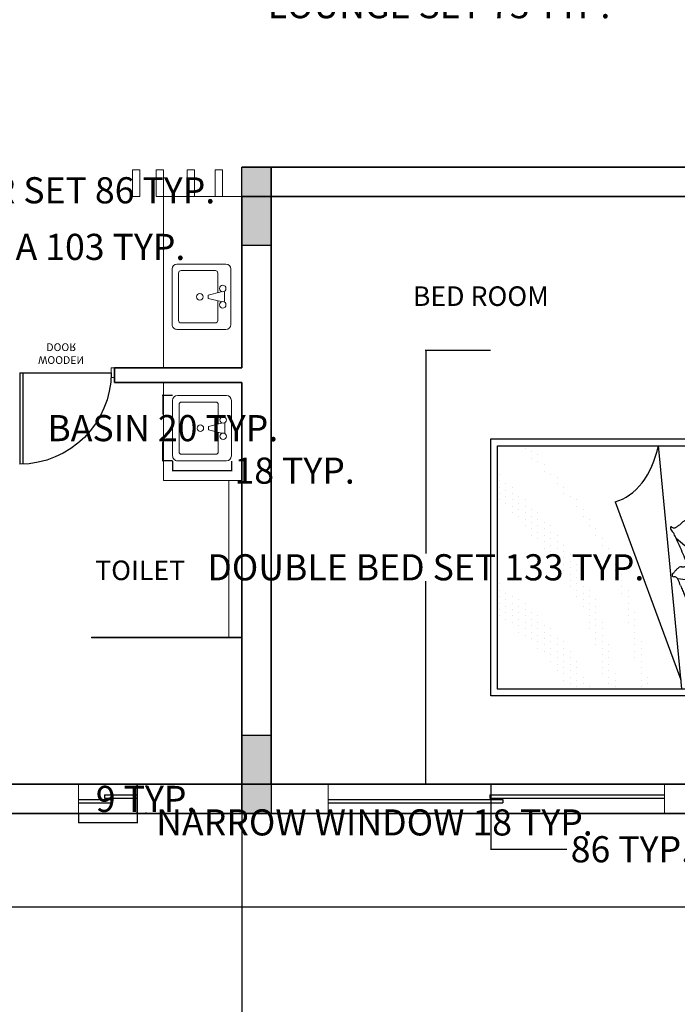
# Model space of a CAD drawing. Units: inches. Extents: x -48 to 50072, y 0 to 21068.
# Tile 63 of 75: x 974 to 1176, y 501 to 803. Entities that reach past the tile are written whole.
import ezdxf

# ---------------------------------------------------------------- set-up
doc = ezdxf.new("R2010")
doc.units = ezdxf.units.IN
doc.header["$MEASUREMENT"] = 0
for name, color, linetype, lineweight in [('A-ANNO-DIMS', 2, 'Continuous', 18), ('A-AREA-IDEN', 7, 'Continuous', 18), ('A-COLS', 1, 'Continuous', 35), ('A-DOOR', 4, 'Continuous', 18), ('A-FLOR-CASE', 9, 'Continuous', 18), ('A-FLOR-FIXT', 4, 'Continuous', 18), ('A-FLOR-SCRN', 32, 'Continuous', 18), ('A-GLAZ', 4, 'Continuous', 18), ('A-WALL', 7, 'Continuous', 35), ('FURNITURE', 44, 'Continuous', 18)]:
    doc.layers.add(name, color=color, linetype=linetype, lineweight=lineweight)
doc.layers.add('Layer3', color=176, linetype='Continuous')
doc.styles.get("Standard").update_dxf_attribs({"font": 'arial.ttf'})
doc.dimstyles.get("Standard").update_dxf_attribs({"dimtxt": 8, "dimasz": 0.18, "dimexe": 0.18, "dimexo": 0.0625, "dimgap": 0.09, "dimtad": 0, "dimtih": 1, "dimtoh": 1, "dimdec": 1, "dimzin": 0, "dimdsep": 46, "dimlunit": 4, "dimtxsty": 'Standard', "dimblk": 'ARCHTICK', "dimcen": 0.09, "dimadec": 0, "dimazin": 0, "dimtfac": 1, "dimtdec": 1, "dimtofl": 0, "dimtmove": 0, "dimatfit": 3, "dimldrblk": 'ARCHTICK', "dimfxl": 1, "dimtolj": 1, "dimtzin": 0, "dimarcsym": 0})

# ---------------------------------------------------------------- blocks, each defined once
blk = doc.blocks.new('bnniku')
at = {"layer": 'Defpoints'}
h = blk.add_hatch(color=256, dxfattribs=at)
h.dxf.hatch_style = 1
h.paths.add_polyline_path([(767.55, 1114.04), (758.55, 1114.04), (758.55, 1090.04), (767.55, 1090.04)])
for p, q in [((758.55, 1114.04), (767.55, 1114.04)), ((758.55, 1090.04), (758.55, 1114.04)), ((767.55, 1114.04), (767.55, 1090.04)), ((767.55, 1090.04), (758.55, 1090.04))]:
    blk.add_line(p, q, dxfattribs=at)
blk = doc.blocks.new('gthyerhy')
at = {"layer": 'Defpoints'}
for p, q in [((665.59, 603.33), (665.59, 631.33)), ((666.59, 603.33), (666.59, 631.32)), ((665.59, 603.33), (693.59, 603.33))]:
    blk.add_line(p, q, dxfattribs=at)
blk.add_arc((665.59, 603.33), 28, 0, 90, dxfattribs=at)
at = {"insert": (674.82, 600.63), "char_height": 2.3647, "attachment_point": 1}
blk.add_mtext_dynamic_manual_height_columns('\\pxqc;WOODEN ^JDOOR', width=6.8949, gutter_width=11.82, heights=[0], dxfattribs=at)
blk = doc.blocks.new('jyugcli')
for p, q in [((342.02, 1025.77), (342.02, 1034.77)), ((360.02, 1025.77), (360.02, 1034.77))]:
    blk.add_line(p, q)
at = {"layer": 'Defpoints'}
for p, q in [((350.02, 1031.47), (360.02, 1031.47)), ((350.02, 1031.47), (350.02, 1030.47)), ((342.02, 1030.07), (352.02, 1030.07)), ((342.02, 1029.07), (352.02, 1029.07)), ((350.02, 1030.47), (360.02, 1030.47)), ((352.02, 1030.07), (352.02, 1029.07))]:
    blk.add_line(p, q, dxfattribs=at)
at = {"layer": 'Layer3'}
for p, q in [((342.02, 1034.77), (360.02, 1034.77)), ((342.02, 1025.77), (360.02, 1025.77))]:
    blk.add_line(p, q, dxfattribs=at)
blk = doc.blocks.new('fdsghhhhhhygr')
for p, q in [((41.77, 686.77), (41.77, 677.77)), ((144.77, 677.77), (144.77, 686.77))]:
    blk.add_line(p, q)
at = {"layer": 'Defpoints'}
for p, q in [((41.77, 682.07), (95.27, 682.07)), ((91.27, 683.47), (144.77, 683.47)), ((91.27, 683.47), (91.27, 682.47)), ((91.27, 682.47), (144.77, 682.47)), ((95.27, 682.07), (95.27, 681.07)), ((41.77, 681.07), (95.27, 681.07))]:
    blk.add_line(p, q, dxfattribs=at)
at = {"layer": 'Layer3'}
for p, q in [((41.77, 686.77), (144.77, 686.77)), ((144.77, 677.77), (41.77, 677.77))]:
    blk.add_line(p, q, dxfattribs=at)
blk = doc.blocks.new('nhrygfdu7yu')
at = {"layer": 'Defpoints'}
for p, q in [((1019.17, 828.61), (845.97, 828.61)), ((845.97, 801.61), (845.97, 828.61)), ((848.67, 804.31), (848.67, 828.61)), ((881.27, 716.83), (881.27, 828.61)), ((884.03, 719.53), (884.03, 827.53)), ((884.03, 827.53), (981.17, 827.53)), ((981.17, 827.53), (981.17, 719.53)), ((983.87, 828.61), (983.87, 716.83)), ((1000.24, 805.98), (1000.24, 825.78)), ((1016.47, 804.31), (1016.47, 828.61)), ((1019.17, 801.61), (1019.17, 828.61)), ((864.18, 805.04), (864.18, 824.84)), ((892.12, 822.13), (892.12, 801.97)), ((929.67, 822.13), (892.12, 822.13)), ((929.67, 822.13), (929.67, 801.78)), ((935.52, 822.13), (935.52, 801.78)), ((935.52, 822.13), (973.07, 822.13)), ((973.07, 822.13), (973.07, 801.97)), ((926.47, 818.07), (927.21, 812.5)), ((947.88, 818.06), (943.61, 812.45)), ((874.65, 814.99), (853.09, 814.99)), ((1010.72, 815.93), (989.15, 815.93)), ((914.58, 810.18), (913.28, 809.99)), ((919.69, 808.14), (914.58, 810.18)), ((927.21, 812.5), (925.82, 805.91)), ((934.43, 807.75), (933.36, 812.55)), ((943.61, 812.45), (939.55, 805.41)), ((923.4, 803.12), (919.69, 808.14)), ((935.49, 804.66), (934.43, 807.75)), ((881.07, 804.31), (848.67, 804.31)), ((881.07, 804.31), (881.07, 804.31)), ((910.77, 803.49), (910.59, 803.15)), ((916.07, 804.42), (910.77, 803.49)), ((919.78, 804.61), (916.07, 804.42)), ((923.4, 803.12), (919.78, 804.61)), ((925.82, 805.91), (923.4, 803.12)), ((923.4, 803.12), (925.08, 798.67)), ((923.4, 803.12), (933.44, 802.1)), ((933.44, 802.1), (936.13, 800.15)), ((935.45, 803.17), (936.69, 800.13)), ((938.59, 802.42), (935.49, 804.66)), ((938.59, 802.42), (937.95, 797.34)), ((939.55, 805.41), (938.59, 802.42)), ((938.59, 802.42), (945.53, 804.13)), ((938.59, 802.42), (941.26, 799.01)), ((945.53, 804.13), (951.08, 803.38)), ((951.08, 803.38), (953.02, 802.3)), ((984.07, 804.31), (1016.47, 804.31)), ((984.07, 804.31), (984.07, 804.31)), ((881.07, 801.61), (845.97, 801.61)), ((884.06, 801.97), (981.18, 801.97)), ((925.08, 798.67), (923.96, 794.21)), ((936.13, 800.15), (936.78, 799.69)), ((936.69, 800.13), (937.65, 797.78)), ((941.26, 799.01), (944.78, 796.45)), ((984.07, 801.61), (1019.17, 801.61)), ((923.96, 794.21), (921.07, 790.83)), ((937.86, 796.54), (937.22, 791.44)), ((944.78, 796.45), (949.8, 796.45)), ((981.13, 793.06), (883.98, 783.7)), ((906.36, 766.47), (977.44, 792.73)), ((976.41, 779.36), (976.41, 779.36)), ((978.98, 779.36), (978.98, 779.36)), ((962.27, 776.79), (962.27, 776.79)), ((964.84, 776.79), (964.84, 776.79)), ((967.41, 776.79), (967.41, 776.79)), ((969.98, 776.79), (969.98, 776.79)), ((972.55, 776.79), (972.55, 776.79)), ((975.13, 776.79), (975.13, 776.79)), ((977.7, 776.79), (977.7, 776.79)), ((980.27, 776.79), (980.27, 776.79)), ((941.69, 771.64), (941.69, 771.64)), ((944.27, 771.64), (944.27, 771.64)), ((946.84, 771.64), (946.84, 771.64)), ((949.41, 771.64), (949.41, 771.64)), ((950.69, 774.21), (950.69, 774.21)), ((951.98, 771.64), (951.98, 771.64)), ((953.27, 774.21), (953.27, 774.21)), ((954.55, 771.64), (954.55, 771.64)), ((955.84, 774.21), (955.84, 774.21)), ((958.41, 774.21), (958.41, 774.21)), ((960.98, 774.21), (960.98, 774.21)), ((963.55, 774.21), (963.55, 774.21)), ((966.13, 774.21), (966.13, 774.21)), ((968.7, 774.21), (968.7, 774.21)), ((935.26, 769.07), (935.26, 769.07)), ((937.84, 769.07), (937.84, 769.07)), ((940.41, 769.07), (940.41, 769.07)), ((942.98, 769.07), (942.98, 769.07)), ((924.98, 763.93), (924.98, 763.93)), ((927.55, 763.93), (927.55, 763.93)), ((928.83, 766.5), (928.83, 766.5)), ((930.12, 763.93), (930.12, 763.93)), ((931.41, 766.5), (931.41, 766.5)), ((933.98, 766.5), (933.98, 766.5)), ((936.55, 766.5), (936.55, 766.5)), ((963.55, 763.93), (963.55, 763.93)), ((966.13, 763.93), (966.13, 763.93)), ((968.7, 763.93), (968.7, 763.93)), ((971.27, 763.93), (971.27, 763.93)), ((973.84, 763.93), (973.84, 763.93)), ((975.13, 766.5), (975.13, 766.5)), ((976.41, 763.93), (976.41, 763.93)), ((977.7, 766.5), (977.7, 766.5)), ((978.98, 763.93), (978.98, 763.93)), ((980.27, 766.5), (980.27, 766.5)), ((921.12, 761.35), (921.12, 761.35)), ((923.69, 761.35), (923.69, 761.35)), ((954.55, 761.35), (954.55, 761.35)), ((957.12, 761.35), (957.12, 761.35)), ((959.7, 761.35), (959.7, 761.35)), ((962.27, 761.35), (962.27, 761.35)), ((964.84, 761.35), (964.84, 761.35)), ((967.41, 761.35), (967.41, 761.35)), ((969.98, 761.35), (969.98, 761.35)), ((972.55, 761.35), (972.55, 761.35)), ((975.13, 761.35), (975.13, 761.35)), ((913.4, 756.21), (913.4, 756.21)), ((915.98, 756.21), (915.98, 756.21)), ((917.26, 758.78), (917.26, 758.78)), ((919.83, 758.78), (919.83, 758.78)), ((941.69, 756.21), (941.69, 756.21)), ((944.27, 756.21), (944.27, 756.21)), ((945.55, 758.78), (945.55, 758.78)), ((946.84, 756.21), (946.84, 756.21)), ((948.12, 758.78), (948.12, 758.78)), ((949.41, 756.21), (949.41, 756.21)), ((950.69, 758.78), (950.69, 758.78)), ((951.98, 756.21), (951.98, 756.21)), ((953.27, 758.78), (953.27, 758.78)), ((954.55, 756.21), (954.55, 756.21)), ((955.84, 758.78), (955.84, 758.78)), ((957.12, 756.21), (957.12, 756.21)), ((958.41, 758.78), (958.41, 758.78)), ((960.98, 758.78), (960.98, 758.78)), ((963.55, 758.78), (963.55, 758.78)), ((980.27, 756.21), (980.27, 756.21)), ((905.69, 751.07), (905.69, 751.07)), ((908.26, 751.07), (908.26, 751.07)), ((909.55, 753.64), (909.55, 753.64)), ((912.12, 753.64), (912.12, 753.64)), ((931.41, 751.07), (931.41, 751.07)), ((933.98, 751.07), (933.98, 751.07)), ((935.26, 753.64), (935.26, 753.64)), ((936.55, 751.07), (936.55, 751.07)), ((937.84, 753.64), (937.84, 753.64)), ((939.12, 751.07), (939.12, 751.07)), ((940.41, 753.64), (940.41, 753.64)), ((941.69, 751.07), (941.69, 751.07)), ((942.98, 753.64), (942.98, 753.64)), ((944.27, 751.07), (944.27, 751.07)), ((945.55, 753.64), (945.55, 753.64)), ((948.12, 753.64), (948.12, 753.64)), ((969.98, 751.07), (969.98, 751.07)), ((972.55, 751.07), (972.55, 751.07)), ((975.13, 751.07), (975.13, 751.07)), ((976.41, 753.64), (976.41, 753.64)), ((977.7, 751.07), (977.7, 751.07)), ((978.98, 753.64), (978.98, 753.64)), ((980.27, 751.07), (980.27, 751.07)), ((904.4, 748.5), (904.4, 748.5)), ((927.55, 748.5), (927.55, 748.5)), ((930.12, 748.5), (930.12, 748.5)), ((932.69, 748.5), (932.69, 748.5)), ((935.26, 748.5), (935.26, 748.5)), ((937.84, 748.5), (937.84, 748.5)), ((940.41, 748.5), (940.41, 748.5)), ((966.13, 748.5), (966.13, 748.5)), ((968.7, 748.5), (968.7, 748.5)), ((971.27, 748.5), (971.27, 748.5)), ((973.84, 748.5), (973.84, 748.5)), ((976.41, 748.5), (976.41, 748.5)), ((978.98, 748.5), (978.98, 748.5)), ((896.69, 743.35), (896.69, 743.35)), ((899.26, 743.35), (899.26, 743.35)), ((900.55, 745.92), (900.55, 745.92)), ((903.12, 745.92), (903.12, 745.92)), ((919.83, 743.35), (919.83, 743.35)), ((922.41, 743.35), (922.41, 743.35)), ((923.69, 745.92), (923.69, 745.92)), ((924.98, 743.35), (924.98, 743.35)), ((926.26, 745.92), (926.26, 745.92)), ((927.55, 743.35), (927.55, 743.35)), ((928.83, 745.92), (928.83, 745.92)), ((930.12, 743.35), (930.12, 743.35)), ((931.41, 745.92), (931.41, 745.92)), ((932.69, 743.35), (932.69, 743.35)), ((933.98, 745.92), (933.98, 745.92)), ((960.98, 743.35), (960.98, 743.35)), ((962.27, 745.92), (962.27, 745.92)), ((963.55, 743.35), (963.55, 743.35)), ((964.84, 745.92), (964.84, 745.92)), ((966.13, 743.35), (966.13, 743.35)), ((967.41, 745.92), (967.41, 745.92)), ((968.7, 743.35), (968.7, 743.35)), ((969.98, 745.92), (969.98, 745.92)), ((971.27, 743.35), (971.27, 743.35)), ((972.55, 745.92), (972.55, 745.92)), ((973.84, 743.35), (973.84, 743.35)), ((975.13, 745.92), (975.13, 745.92)), ((977.7, 745.92), (977.7, 745.92)), ((895.4, 740.78), (895.4, 740.78)), ((915.98, 740.78), (915.98, 740.78)), ((918.55, 740.78), (918.55, 740.78)), ((921.12, 740.78), (921.12, 740.78)), ((923.69, 740.78), (923.69, 740.78)), ((926.26, 740.78), (926.26, 740.78)), ((928.83, 740.78), (928.83, 740.78)), ((957.12, 740.78), (957.12, 740.78)), ((959.7, 740.78), (959.7, 740.78)), ((962.27, 740.78), (962.27, 740.78)), ((964.84, 740.78), (964.84, 740.78)), ((967.41, 740.78), (967.41, 740.78)), ((969.98, 740.78), (969.98, 740.78)), ((887.69, 735.64), (887.69, 735.64)), ((890.26, 735.64), (890.26, 735.64)), ((891.54, 738.21), (891.54, 738.21)), ((894.12, 738.21), (894.12, 738.21)), ((910.83, 735.64), (910.83, 735.64)), ((913.4, 735.64), (913.4, 735.64)), ((914.69, 738.21), (914.69, 738.21)), ((915.98, 735.64), (915.98, 735.64)), ((917.26, 738.21), (917.26, 738.21)), ((918.55, 735.64), (918.55, 735.64)), ((919.83, 738.21), (919.83, 738.21)), ((921.12, 735.64), (921.12, 735.64)), ((922.41, 738.21), (922.41, 738.21)), ((924.98, 738.21), (924.98, 738.21)), ((951.98, 735.64), (951.98, 735.64)), ((954.55, 735.64), (954.55, 735.64)), ((955.84, 738.21), (955.84, 738.21)), ((957.12, 735.64), (957.12, 735.64)), ((958.41, 738.21), (958.41, 738.21)), ((959.7, 735.64), (959.7, 735.64)), ((960.98, 738.21), (960.98, 738.21)), ((962.27, 735.64), (962.27, 735.64)), ((963.55, 738.21), (963.55, 738.21)), ((964.84, 735.64), (964.84, 735.64)), ((966.13, 738.21), (966.13, 738.21)), ((886.4, 733.07), (886.4, 733.07)), ((888.97, 733.07), (888.97, 733.07)), ((909.55, 733.07), (909.55, 733.07)), ((912.12, 733.07), (912.12, 733.07)), ((914.69, 733.07), (914.69, 733.07)), ((917.26, 733.07), (917.26, 733.07)), ((919.83, 733.07), (919.83, 733.07)), ((950.69, 733.07), (950.69, 733.07)), ((953.27, 733.07), (953.27, 733.07)), ((955.84, 733.07), (955.84, 733.07)), ((958.41, 733.07), (958.41, 733.07)), ((960.98, 733.07), (960.98, 733.07)), ((885.12, 730.49), (885.12, 730.49)), ((904.4, 727.92), (904.4, 727.92)), ((905.69, 730.49), (905.69, 730.49)), ((906.97, 727.92), (906.97, 727.92)), ((908.26, 730.49), (908.26, 730.49)), ((909.55, 727.92), (909.55, 727.92)), ((910.83, 730.49), (910.83, 730.49)), ((912.12, 727.92), (912.12, 727.92)), ((913.4, 730.49), (913.4, 730.49)), ((915.98, 730.49), (915.98, 730.49)), ((945.55, 727.92), (945.55, 727.92)), ((946.84, 730.49), (946.84, 730.49)), ((948.12, 727.92), (948.12, 727.92)), ((949.41, 730.49), (949.41, 730.49)), ((950.69, 727.92), (950.69, 727.92)), ((951.98, 730.49), (951.98, 730.49)), ((953.27, 727.92), (953.27, 727.92)), ((954.55, 730.49), (954.55, 730.49)), ((955.84, 727.92), (955.84, 727.92)), ((957.12, 730.49), (957.12, 730.49)), ((958.41, 727.92), (958.41, 727.92)), ((959.7, 730.49), (959.7, 730.49)), ((900.55, 725.35), (900.55, 725.35)), ((903.12, 725.35), (903.12, 725.35)), ((905.69, 725.35), (905.69, 725.35)), ((908.26, 725.35), (908.26, 725.35)), ((910.83, 725.35), (910.83, 725.35)), ((944.27, 725.35), (944.27, 725.35)), ((946.84, 725.35), (946.84, 725.35)), ((949.41, 725.35), (949.41, 725.35)), ((951.98, 725.35), (951.98, 725.35)), ((954.55, 725.35), (954.55, 725.35)), ((981.17, 719.53), (884.03, 719.53)), ((895.4, 720.21), (895.4, 720.21)), ((897.97, 720.21), (897.97, 720.21)), ((899.26, 722.78), (899.26, 722.78)), ((900.55, 720.21), (900.55, 720.21)), ((901.83, 722.78), (901.83, 722.78)), ((903.12, 720.21), (903.12, 720.21)), ((904.4, 722.78), (904.4, 722.78)), ((905.69, 720.21), (905.69, 720.21)), ((906.97, 722.78), (906.97, 722.78)), ((939.12, 720.21), (939.12, 720.21)), ((941.69, 720.21), (941.69, 720.21)), ((942.98, 722.78), (942.98, 722.78)), ((944.27, 720.21), (944.27, 720.21)), ((945.55, 722.78), (945.55, 722.78)), ((946.84, 720.21), (946.84, 720.21)), ((948.12, 722.78), (948.12, 722.78)), ((949.41, 720.21), (949.41, 720.21)), ((950.69, 722.78), (950.69, 722.78)), ((951.98, 720.21), (951.98, 720.21)), ((953.27, 722.78), (953.27, 722.78)), ((983.87, 716.83), (881.27, 716.83))]:
    blk.add_line(p, q, dxfattribs=at)
for centre, radius in [((864.18, 814.99), 8.1), ((1000.24, 815.93), 8.1), ((1000.24, 815.93), 6.48), ((864.18, 814.99), 6.48)]:
    blk.add_circle(centre, radius, dxfattribs=at)
for centre, radius, start, end in [((926.67, 817.58), 0.687, 51.1864, 183.2455), ((924.75, 815.18), 3.76, 45.8726, 51.1864), ((929.07, 819.63), 2.44, 225.8726, 232.4713), ((948.22, 814.9), 3.25, 110.3452, 128.5854), ((947.75, 816.16), 1.9, 86.0516, 110.3452), ((947.87, 817.82), 0.239, 13.2808, 86.0516), ((947.77, 817.8), 0.34, 306.5792, 13.2808), ((971.1, 717.04), 108.88, 116.4147, 117.4999), ((848.26, 964.34), 167.25, 296.4147, 297.2902), ((924.05, 817.43), 1.94, 297.2902, 3.2455), ((940.16, 834.08), 20.66, 232.4713, 233.7837), ((906.88, 788.64), 35.67, 52.7849, 53.7837), ((921.35, 807.68), 11.75, 46.4776, 52.7849), ((926.56, 813.17), 4.18, 35.8936, 46.4776), ((928.96, 814.91), 1.22, 351.9508, 35.8936), ((932.62, 814.39), 2.47, 171.9508, 202.4162), ((883.03, 974.91), 169.83, 286.6085, 289.0836), ((848.62, 1074.38), 275.09, 289.0836, 290.1287), ((927.73, 858.54), 45.2, 290.1287, 292.7069), ((943.53, 820.78), 4.28, 292.7069, 308.5854), ((951.77, 816.3), 4.17, 169.5926, 177.2714), ((948.44, 816.46), 0.826, 177.2714, 194.5709), ((949.69, 816.78), 2.12, 194.5709, 206.8179), ((948.43, 816.91), 0.765, 126.5792, 169.5926), ((964.76, 824.4), 19.01, 206.8179, 210.9056), ((957.44, 820.02), 10.47, 210.9056, 219.7005), ((905.47, 831.87), 23.22, 282.6252, 290.7486), ((901.77, 841.65), 33.68, 290.7486, 297.4921), ((771.78, 1091.44), 315.27, 297.4921, 297.8482), ((1072.97, 521.35), 329.5, 117.4999, 117.8482), ((980.52, 834.15), 54.29, 202.4162, 205.0529), ((929.77, 818.2), 6.29, 280.7366, 286.6085), ((1013.86, 849.73), 91.09, 205.0529, 207.0884), ((946.01, 810.53), 4.37, 26.0735, 39.7005), ((940.41, 807.79), 10.61, 17.8396, 26.0735), ((847.55, 777.91), 108.16, 15.2625, 17.8396), ((908.02, 808.45), 0.313, 121.6917, 179.0386), ((908.61, 808.44), 0.905, 179.0386, 229.4914), ((909.3, 806.38), 2.75, 103.0402, 121.6917), ((905.38, 804.66), 4.08, 26.3332, 49.4914), ((909.41, 805.91), 3.23, 86.6119, 103.0402), ((780.21, 742.7), 143.74, 25.1732, 26.3332), ((909.8, 812.53), 3.4, 266.6119, 282.6252), ((1008.01, 846.74), 84.52, 207.0884, 209.936), ((866.04, 782.95), 89, 13.841, 15.2625), ((901.51, 799.71), 9.71, 20.7081, 25.1732), ((883.04, 792.73), 29.45, 18.2369, 20.7081), ((924.73, 798.79), 11.57, 22.2355, 29.936), ((981.05, 811.29), 29.45, 193.841, 196.3122), ((962.1, 805.74), 9.71, 196.3122, 200.7773), ((1087.42, 853.29), 143.74, 200.7773, 201.9373), ((995.54, 829.8), 89, 198.2369, 199.6584), ((1013.59, 836.25), 108.16, 199.6584, 202.2355), ((957.87, 801.11), 4.08, 201.9373, 225.0955), ((954.35, 797.58), 0.905, 354.6428, 45.0955), ((923.29, 799.33), 10.61, 202.2355, 210.4694), ((993.31, 637.11), 169.83, 111.0043, 113.4795), ((880.68, 777.46), 54.29, 18.0203, 19.3448), ((929.96, 793.49), 2.47, 347.5549, 18.0203), ((934.7, 789.77), 6.29, 98.1216, 111.0043), ((934.31, 792.46), 3.58, 85.4882, 98.1216), ((934.9, 799.87), 3.85, 265.4882, 277.6784), ((934.12, 805.65), 9.69, 277.6784, 284.8807), ((939.32, 786.09), 10.56, 97.9822, 104.8807), ((938.8, 798.25), 1.24, 202.2355, 252.8133), ((938.1, 794.73), 1.83, 85.7407, 97.9822), ((938.28, 797.05), 0.497, 265.7407, 289.3799), ((938.36, 796.82), 0.252, 289.3799, 72.8133), ((1069.09, 504.93), 315.27, 113.0962, 113.4523), ((958.63, 763.95), 33.68, 106.3527, 113.0962), ((955.69, 773.98), 23.22, 98.2293, 106.3527), ((952.85, 793.6), 3.4, 82.216, 98.2293), ((953.75, 800.17), 3.23, 262.216, 278.6443), ((953.82, 799.69), 2.75, 278.6443, 297.2959), ((954.94, 797.53), 0.313, 297.2959, 354.6428), ((917.92, 796.17), 4.37, 210.4694, 224.0964), ((907.26, 785.84), 10.47, 35.3015, 44.0964), ((900.29, 780.91), 19.01, 31.2138, 35.3015), ((914.73, 789.66), 2.12, 18.9668, 31.2138), ((915.96, 790.08), 0.826, 1.6673, 18.9668), ((939.83, 749.71), 45.2, 114.5246, 117.1028), ((1035.25, 540.56), 275.09, 113.4795, 114.5246), ((933.57, 792.7), 1.22, 167.5549, 211.4977), ((936.09, 794.24), 4.18, 211.4977, 222.0817), ((941.71, 799.32), 11.75, 222.0817, 228.389), ((957.59, 817.2), 35.67, 228.389, 229.3878), ((938.27, 789.81), 1.94, 112.8944, 178.8496), ((1002.58, 637.52), 167.25, 112.0188, 112.8944), ((899.06, 893.51), 108.88, 292.0188, 293.104), ((812.48, 1096.43), 329.5, 293.104, 293.4523), ((916.73, 788.79), 0.34, 130.9751, 197.6767), ((916.63, 788.76), 0.239, 197.6767, 270.4475), ((916, 789.63), 0.765, 310.9751, 353.9885), ((916.62, 790.42), 1.9, 270.4475, 294.7411), ((912.62, 789.98), 4.17, 353.9885, 1.6673), ((916.05, 791.65), 3.25, 294.7411, 312.9813), ((921.18, 786.14), 4.28, 117.1028, 132.9813), ((920.93, 774.44), 20.66, 48.0754, 49.3878), ((933.1, 787.99), 2.44, 41.4767, 48.0754), ((937.75, 792.1), 3.76, 221.4767, 226.7905), ((935.64, 789.86), 0.687, 226.7905, 358.8496)]:
    blk.add_arc(centre, radius, start, end, dxfattribs=at)
blk.add_ellipse((874.1, 762.91), major_axis=(32.71, 0), ratio=0.667085, start_param=0.16392, end_param=1.263761, dxfattribs=at)
blk = doc.blocks.new('A$C329C6BD7')
at = {"linetype": 'ByBlock'}
for p, q in [((0, 0.4191), (0, 0.0381)), ((0.4699, 0.4572), (0.0381, 0.4572)), ((0.2159, 0.4064), (0.2921, 0.4064)), ((0.508, 0.0381), (0.508, 0.4191)), ((0.0508, 0.0698), (0.0508, 0.3365)), ((0.0698, 0.3556), (0.2223, 0.3556)), ((0.2159, 0.381), (0.2413, 0.2794)), ((0.2667, 0.2794), (0.2921, 0.381)), ((0.2858, 0.3556), (0.4382, 0.3556)), ((0.4572, 0.3365), (0.4572, 0.0698)), ((0.2413, 0.2794), (0.2667, 0.2794)), ((0.4382, 0.0508), (0.0698, 0.0508)), ((0.0381, 0), (0.4699, 0))]:
    blk.add_line(p, q, dxfattribs=at)
for centre in [(0.1905, 0.3937), (0.3175, 0.3937), (0.254, 0.2159)]:
    blk.add_circle(centre, 0.0254, dxfattribs=at)
for centre, radius, start, end in [((0.0381, 0.4191), 0.0381, 90, 180), ((0.4699, 0.4191), 0.0381, 0, 90), ((0.0698, 0.3365), 0.0191, 90, 180), ((0.4382, 0.3365), 0.0191, 0, 90), ((0.0381, 0.0381), 0.0381, 180, 270), ((0.0698, 0.0698), 0.0191, 180, 270), ((0.4382, 0.0698), 0.0191, 270, 0), ((0.4699, 0.0381), 0.0381, 270, 0)]:
    blk.add_arc(centre, radius, start, end, dxfattribs=at)
blk = doc.blocks.new('_ArchTick')
at = {"color": 0, "linetype": 'ByBlock', "const_width": 0.15}
blk.add_lwpolyline([(-0.5, -0.5), (0.5, 0.5)], dxfattribs=at)
blk = doc.blocks.new('*D56')
at = {"layer": 'A-ANNO-DIMS', "color": 0, "lineweight": -2, "transparency": 16777216}
for p, q in [((992.26, 559.4), (992.26, 556.58)), ((1010.26, 559.4), (1010.26, 556.58)), ((992.26, 556.76), (1010.26, 556.76)), ((1010.26, 556.76), (1010.44, 556.76))]:
    blk.add_line(p, q, dxfattribs=at)
at = {"layer": 'Defpoints', "color": 0, "transparency": 16777216}
for p in [(992.26, 559.46), (1010.26, 559.46), (1010.26, 556.76)]:
    blk.add_point(p, dxfattribs=at)
at = {"layer": 'A-ANNO-DIMS', "color": 0, "lineweight": -2, "transparency": 16777216, "xscale": 0.18, "yscale": 0.18, "zscale": 0.18, "rotation": 180}
blk.add_blockref('_ArchTick', (992.26, 556.76), dxfattribs=at)
at = {"layer": 'A-ANNO-DIMS', "color": 0, "lineweight": -2, "transparency": 16777216, "xscale": 0.18, "yscale": 0.18, "zscale": 0.18}
blk.add_blockref('_ArchTick', (1010.26, 556.76), dxfattribs=at)
at = {"layer": 'A-ANNO-DIMS', "color": 0, "transparency": 16777216, "insert": (1082.89, 556.76), "char_height": 8, "attachment_point": 5}
blk.add_mtext('\\A1;NARROW WINDOW 18 TYP.', dxfattribs=at)
blk = doc.blocks.new('*D57')
at = {"layer": 'A-ANNO-DIMS', "color": 0, "lineweight": -2, "transparency": 16777216}
for p, q in [((1010.32, 568.46), (1013.14, 568.46)), ((1012.96, 568.46), (1012.96, 568.14)), ((1010.32, 559.46), (1013.14, 559.46)), ((1012.96, 559.46), (1012.96, 559.79))]:
    blk.add_line(p, q, dxfattribs=at)
at = {"layer": 'Defpoints', "color": 0, "transparency": 16777216}
for p in [(1010.26, 568.46), (1012.96, 568.46), (1010.26, 559.46)]:
    blk.add_point(p, dxfattribs=at)
at = {"layer": 'A-ANNO-DIMS', "color": 0, "lineweight": -2, "transparency": 16777216, "xscale": 0.18, "yscale": 0.18, "zscale": 0.18}
for p, rotation in [((1012.96, 568.46), 90), ((1012.96, 559.46), 270)]:
    blk.add_blockref('_ArchTick', p, dxfattribs=dict(at, rotation=rotation))
at = {"layer": 'A-ANNO-DIMS', "color": 0, "transparency": 16777216, "insert": (1012.96, 563.96), "char_height": 8, "attachment_point": 5}
blk.add_mtext('\\A1;9 TYP.', dxfattribs=at)
blk = doc.blocks.new('*D60')
at = {"layer": 'A-ANNO-DIMS', "color": 0, "lineweight": -2, "transparency": 16777216}
for p, q in [((787.01, 748.4), (787.01, 732.83)), ((890.01, 748.4), (890.01, 732.83)), ((787.01, 733.01), (890.01, 733.01)), ((890.01, 733.01), (890.19, 733.01))]:
    blk.add_line(p, q, dxfattribs=at)
at = {"layer": 'Defpoints', "color": 0, "transparency": 16777216}
for p in [(787.01, 748.46), (890.01, 748.46), (890.01, 733.01)]:
    blk.add_point(p, dxfattribs=at)
at = {"layer": 'A-ANNO-DIMS', "color": 0, "lineweight": -2, "transparency": 16777216, "xscale": 0.18, "yscale": 0.18, "zscale": 0.18, "rotation": 180}
blk.add_blockref('_ArchTick', (787.01, 733.01), dxfattribs=at)
at = {"layer": 'A-ANNO-DIMS', "color": 0, "lineweight": -2, "transparency": 16777216, "xscale": 0.18, "yscale": 0.18, "zscale": 0.18}
blk.add_blockref('_ArchTick', (890.01, 733.01), dxfattribs=at)
at = {"layer": 'A-ANNO-DIMS', "color": 0, "transparency": 16777216, "insert": (960.35, 733.01), "char_height": 8, "attachment_point": 5}
blk.add_mtext('\\A1;SLIDING DOOR A 103 TYP.', dxfattribs=at)
blk = doc.blocks.new('*D72')
at = {"layer": 'A-ANNO-DIMS', "color": 0, "lineweight": -2, "transparency": 16777216}
for p, q in [((1118.47, 701.3), (1098.43, 701.3)), ((1098.61, 701.3), (1098.61, 639.11)), ((1098.61, 568.46), (1098.61, 630.65)), ((1118.47, 568.46), (1098.43, 568.46))]:
    blk.add_line(p, q, dxfattribs=at)
at = {"layer": 'Defpoints', "color": 0, "transparency": 16777216}
for p in [(1118.53, 701.3), (1098.61, 568.46), (1118.53, 568.46)]:
    blk.add_point(p, dxfattribs=at)
at = {"layer": 'A-ANNO-DIMS', "color": 0, "lineweight": -2, "transparency": 16777216, "xscale": 0.18, "yscale": 0.18, "zscale": 0.18}
for p, rotation in [((1098.61, 701.3), 90), ((1098.61, 568.46), 270)]:
    blk.add_blockref('_ArchTick', p, dxfattribs=dict(at, rotation=rotation))
at = {"layer": 'A-ANNO-DIMS', "color": 0, "transparency": 16777216, "insert": (1098.61, 634.88), "char_height": 8, "attachment_point": 5}
blk.add_mtext('\\A1;DOUBLE BED SET 133 TYP.', dxfattribs=at)
blk = doc.blocks.new('*D73')
at = {"layer": 'A-ANNO-DIMS', "color": 0, "lineweight": -2, "transparency": 16777216}
for p, q in [((1118.53, 568.4), (1118.53, 548.36)), ((1204.26, 568.4), (1204.26, 548.36)), ((1118.53, 548.54), (1141.83, 548.54)), ((1204.26, 548.54), (1180.96, 548.54))]:
    blk.add_line(p, q, dxfattribs=at)
at = {"layer": 'Defpoints', "color": 0, "transparency": 16777216}
for p in [(1118.53, 568.46), (1204.26, 568.46), (1204.26, 548.54)]:
    blk.add_point(p, dxfattribs=at)
at = {"layer": 'A-ANNO-DIMS', "color": 0, "lineweight": -2, "transparency": 16777216, "xscale": 0.18, "yscale": 0.18, "zscale": 0.18, "rotation": 180}
blk.add_blockref('_ArchTick', (1118.53, 548.54), dxfattribs=at)
at = {"layer": 'A-ANNO-DIMS', "color": 0, "lineweight": -2, "transparency": 16777216, "xscale": 0.18, "yscale": 0.18, "zscale": 0.18}
blk.add_blockref('_ArchTick', (1204.26, 548.54), dxfattribs=at)
at = {"layer": 'A-ANNO-DIMS', "color": 0, "transparency": 16777216, "insert": (1161.4, 548.54), "char_height": 8, "attachment_point": 5}
blk.add_mtext('\\A1;86 TYP.', dxfattribs=at)
blk = doc.blocks.new('*D76')
at = {"layer": 'A-ANNO-DIMS', "color": 0, "lineweight": -2, "transparency": 16777216}
for p, q in [((972.12, 817.98), (972.12, 806.85)), ((1045.51, 817.98), (1045.51, 806.85)), ((972.12, 807.03), (1045.51, 807.03)), ((1045.51, 807.03), (1045.69, 807.03))]:
    blk.add_line(p, q, dxfattribs=at)
at = {"layer": 'Defpoints', "color": 0, "transparency": 16777216}
for p in [(972.12, 818.04), (1045.51, 818.04), (1045.51, 807.03)]:
    blk.add_point(p, dxfattribs=at)
at = {"layer": 'A-ANNO-DIMS', "color": 0, "lineweight": -2, "transparency": 16777216, "xscale": 0.18, "yscale": 0.18, "zscale": 0.18, "rotation": 180}
blk.add_blockref('_ArchTick', (972.12, 807.03), dxfattribs=at)
at = {"layer": 'A-ANNO-DIMS', "color": 0, "lineweight": -2, "transparency": 16777216, "xscale": 0.18, "yscale": 0.18, "zscale": 0.18}
blk.add_blockref('_ArchTick', (1045.51, 807.03), dxfattribs=at)
at = {"layer": 'A-ANNO-DIMS', "color": 0, "transparency": 16777216, "insert": (1102.65, 807.03), "char_height": 8, "attachment_point": 5}
blk.add_mtext('\\A1;LOUNGE SET 73 TYP.', dxfattribs=at)
blk = doc.blocks.new('*D86')
at = {"layer": 'A-ANNO-DIMS', "color": 0, "lineweight": -2, "transparency": 16777216}
for p, q in [((1021.01, 687.5), (1017.89, 687.5)), ((1018.07, 687.5), (1018.07, 681.72)), ((1018.07, 667.49), (1018.07, 673.27)), ((1021.01, 667.49), (1017.89, 667.49))]:
    blk.add_line(p, q, dxfattribs=at)
at = {"layer": 'Defpoints', "color": 0, "transparency": 16777216}
for p in [(1021.07, 687.5), (1018.07, 667.49), (1021.07, 667.49)]:
    blk.add_point(p, dxfattribs=at)
at = {"layer": 'A-ANNO-DIMS', "color": 0, "lineweight": -2, "transparency": 16777216, "xscale": 0.18, "yscale": 0.18, "zscale": 0.18}
for p, rotation in [((1018.07, 687.5), 90), ((1018.07, 667.49), 270)]:
    blk.add_blockref('_ArchTick', p, dxfattribs=dict(at, rotation=rotation))
at = {"layer": 'A-ANNO-DIMS', "color": 0, "transparency": 16777216, "insert": (1018.07, 677.5), "char_height": 8, "attachment_point": 5}
blk.add_mtext('\\A1;BASIN 20 TYP.', dxfattribs=at)
blk = doc.blocks.new('*D87')
at = {"layer": 'A-ANNO-DIMS', "color": 0, "lineweight": -2, "transparency": 16777216}
for p, q in [((1021.07, 667.43), (1021.07, 664.31)), ((1039.08, 667.43), (1039.08, 664.31)), ((1021.07, 664.49), (1039.08, 664.49)), ((1039.08, 664.49), (1039.26, 664.49))]:
    blk.add_line(p, q, dxfattribs=at)
at = {"layer": 'Defpoints', "color": 0, "transparency": 16777216}
for p in [(1021.07, 667.49), (1039.08, 667.49), (1039.08, 664.49)]:
    blk.add_point(p, dxfattribs=at)
at = {"layer": 'A-ANNO-DIMS', "color": 0, "lineweight": -2, "transparency": 16777216, "xscale": 0.18, "yscale": 0.18, "zscale": 0.18, "rotation": 180}
blk.add_blockref('_ArchTick', (1021.07, 664.49), dxfattribs=at)
at = {"layer": 'A-ANNO-DIMS', "color": 0, "lineweight": -2, "transparency": 16777216, "xscale": 0.18, "yscale": 0.18, "zscale": 0.18}
blk.add_blockref('_ArchTick', (1039.08, 664.49), dxfattribs=at)
at = {"layer": 'A-ANNO-DIMS', "color": 0, "transparency": 16777216, "insert": (1058.44, 664.49), "char_height": 8, "attachment_point": 5}
blk.add_mtext('\\A1;18 TYP.', dxfattribs=at)
blk = doc.blocks.new('*D98')
at = {"layer": 'A-ANNO-DIMS', "color": 0, "lineweight": -2, "transparency": 16777216}
for p, q in [((957.32, 793.46), (970.38, 793.46)), ((970.2, 793.46), (970.2, 754.56)), ((970.2, 707.21), (970.2, 746.11)), ((957.32, 707.21), (970.38, 707.21))]:
    blk.add_line(p, q, dxfattribs=at)
at = {"layer": 'Defpoints', "color": 0, "transparency": 16777216}
for p in [(957.26, 793.46), (970.2, 793.46), (957.26, 707.21)]:
    blk.add_point(p, dxfattribs=at)
at = {"layer": 'A-ANNO-DIMS', "color": 0, "lineweight": -2, "transparency": 16777216, "xscale": 0.18, "yscale": 0.18, "zscale": 0.18}
for p, rotation in [((970.2, 793.46), 90), ((970.2, 707.21), 270)]:
    blk.add_blockref('_ArchTick', p, dxfattribs=dict(at, rotation=rotation))
at = {"layer": 'A-ANNO-DIMS', "color": 0, "transparency": 16777216, "insert": (970.2, 750.34), "char_height": 8, "attachment_point": 5}
blk.add_mtext('\\A1;ENTRY DOOR SET 86 TYP.', dxfattribs=at)
blk = doc.blocks.new('*D137')
at = {"layer": 'A-ANNO-DIMS', "color": 0, "lineweight": -2, "transparency": 16777216}
for p, q in [((961.26, 559.4), (961.26, 236.63)), ((1042.26, 559.4), (1042.26, 236.63)), ((961.26, 236.81), (996.71, 236.81)), ((1042.26, 236.81), (1006.81, 236.81))]:
    blk.add_line(p, q, dxfattribs=at)
at = {"layer": 'Defpoints', "color": 0, "transparency": 16777216}
for p in [(961.26, 559.46), (1042.26, 559.46), (1042.26, 236.81)]:
    blk.add_point(p, dxfattribs=at)
at = {"layer": 'A-ANNO-DIMS', "color": 0, "lineweight": -2, "transparency": 16777216, "xscale": 0.18, "yscale": 0.18, "zscale": 0.18, "rotation": 180}
blk.add_blockref('_ArchTick', (961.26, 236.81), dxfattribs=at)
at = {"layer": 'A-ANNO-DIMS', "color": 0, "lineweight": -2, "transparency": 16777216, "xscale": 0.18, "yscale": 0.18, "zscale": 0.18}
blk.add_blockref('_ArchTick', (1042.26, 236.81), dxfattribs=at)
at = {"layer": 'A-ANNO-DIMS', "color": 0, "transparency": 16777216, "insert": (1001.76, 236.81), "char_height": 8, "attachment_point": 5}
blk.add_mtext('\\A1;81', dxfattribs=at)
blk = doc.blocks.new('*D138')
at = {"layer": 'A-ANNO-DIMS', "color": 0, "lineweight": -2, "transparency": 16777216}
for p, q in [((1042.26, 559.4), (1042.26, 236.63)), ((1208.76, 559.4), (1208.76, 236.63)), ((1042.26, 236.81), (1112.27, 236.81)), ((1208.76, 236.81), (1138.75, 236.81))]:
    blk.add_line(p, q, dxfattribs=at)
at = {"layer": 'Defpoints', "color": 0, "transparency": 16777216}
for p in [(1042.26, 559.46), (1208.76, 559.46), (1208.76, 236.81)]:
    blk.add_point(p, dxfattribs=at)
at = {"layer": 'A-ANNO-DIMS', "color": 0, "lineweight": -2, "transparency": 16777216, "xscale": 0.18, "yscale": 0.18, "zscale": 0.18, "rotation": 180}
blk.add_blockref('_ArchTick', (1042.26, 236.81), dxfattribs=at)
at = {"layer": 'A-ANNO-DIMS', "color": 0, "lineweight": -2, "transparency": 16777216, "xscale": 0.18, "yscale": 0.18, "zscale": 0.18}
blk.add_blockref('_ArchTick', (1208.76, 236.81), dxfattribs=at)
at = {"layer": 'A-ANNO-DIMS', "color": 0, "transparency": 16777216, "insert": (1125.51, 236.81), "char_height": 8, "attachment_point": 5}
blk.add_mtext('\\A1;166.5', dxfattribs=at)
blk = doc.blocks.new('*D146')
at = {"layer": 'A-ANNO-DIMS', "color": 0, "lineweight": -2, "transparency": 16777216}
for p, q in [((1208.7, 559.46), (710.63, 559.46)), ((710.81, 559.46), (710.81, 549.29)), ((710.81, 530.76), (710.81, 540.94)), ((1208.7, 530.76), (710.63, 530.76))]:
    blk.add_line(p, q, dxfattribs=at)
at = {"layer": 'Defpoints', "color": 0, "transparency": 16777216}
for p in [(710.81, 559.46), (1208.76, 559.46), (1208.76, 530.76)]:
    blk.add_point(p, dxfattribs=at)
at = {"layer": 'A-ANNO-DIMS', "color": 0, "lineweight": -2, "transparency": 16777216, "xscale": 0.18, "yscale": 0.18, "zscale": 0.18}
for p, rotation in [((710.81, 559.46), 90), ((710.81, 530.76), 270)]:
    blk.add_blockref('_ArchTick', p, dxfattribs=dict(at, rotation=rotation))
at = {"layer": 'A-ANNO-DIMS', "color": 0, "transparency": 16777216, "insert": (710.81, 545.11), "char_height": 8, "attachment_point": 5}
blk.add_mtext('\\A1;28.7', dxfattribs=at)

msp = doc.modelspace()

# ---------------------------------------------------------------- linework, layer by layer
at = {"layer": 'A-DOOR'}
for p, q in [((1002.261, 692.964), (1002.261, 695.964)), ((1002.261, 695.964), (1003.261, 695.964)), ((1002.261, 692.964), (1003.261, 692.964))]:
    msp.add_line(p, q, dxfattribs=at)
at = {"layer": 'A-FLOR-CASE'}
for p, q in [((1018.261, 695.964), (1018.261, 748.464)), ((1018.261, 748.464), (1042.261, 748.464)), ((1018.261, 661.464), (1018.261, 691.464)), ((1042.261, 661.464), (1018.261, 661.464))]:
    msp.add_line(p, q, dxfattribs=at)
at = {"layer": 'A-FLOR-SCRN'}
for points in [[(1011.002, 748.464), (1008.787, 748.464), (1008.787, 756.569), (1011.002, 756.569)], [(1018.261, 748.464), (1016.046, 748.464), (1016.046, 756.569), (1018.261, 756.569)], [(1018.261, 748.464), (1016.046, 748.464), (1016.046, 756.569), (1018.261, 756.569)], [(1018.261, 748.464), (1016.046, 748.464), (1016.046, 756.569), (1018.261, 756.569)], [(1027.745, 748.464), (1025.53, 748.464), (1025.53, 756.569), (1027.745, 756.569)], [(1036.334, 748.464), (1034.119, 748.464), (1034.119, 756.569), (1036.334, 756.569)]]:
    msp.add_lwpolyline(points, close=True, dxfattribs=at)
at = {"layer": 'A-GLAZ'}
for p, q in [((1038.261, 613.464), (1038.261, 661.464)), ((1038.261, 661.464), (1038.261, 613.464)), ((996.261, 613.264), (996.261, 613.464)), ((1042.261, 613.464), (996.261, 613.464)), ((1042.261, 613.264), (996.261, 613.264))]:
    msp.add_line(p, q, dxfattribs=at)
at = {"layer": 'A-WALL'}
for p, q in [((1294.261, 757.464), (1042.261, 757.464)), ((1051.261, 568.464), (1051.261, 757.464)), ((1042.261, 695.964), (1042.261, 748.464)), ((1289.761, 748.464), (1042.261, 748.464)), ((1003.261, 691.464), (1003.261, 695.964)), ((1042.261, 695.964), (1003.261, 695.964)), ((1042.261, 691.464), (1003.261, 691.464)), ((1042.261, 559.464), (1042.261, 691.464)), ((1208.761, 568.464), (961.261, 568.464)), ((1010.261, 559.464), (1010.261, 568.464)), ((1208.761, 559.464), (961.261, 559.464))]:
    msp.add_line(p, q, dxfattribs=at)

# ---------------------------------------------------------------- block references
at = {"layer": 'A-COLS'}
for p in [(283.709, -356.573), (283.709, -530.573)]:
    msp.add_blockref('bnniku', p, dxfattribs=at)
at = {"layer": 'A-DOOR', "xscale": -1, "rotation": 180}
msp.add_blockref('gthyerhy', (308.676, 1297.798), dxfattribs=at)
at = {"layer": 'A-DOOR'}
msp.add_blockref('fdsghhhhhhygr', (1026.958, -118.311), dxfattribs=at)
at = {"layer": 'A-FLOR-FIXT', "xscale": 39.38263526611686, "yscale": 39.38263526611686, "zscale": 39.38263526611686, "rotation": 270}
for p in [(1020.916, 727.743), (1021.072, 687.498)]:
    msp.add_blockref('A$C329C6BD7', p, dxfattribs=at)
at = {"layer": 'A-GLAZ'}
msp.add_blockref('jyugcli', (650.244, -466.311), dxfattribs=at)
at = {"layer": 'FURNITURE', "xscale": 0.7669307891904348, "yscale": 0.7669307891904348, "zscale": 0.7669307891904348, "rotation": 270}
msp.add_blockref('nhrygfdu7yu', (568.778, 1350.095), dxfattribs=at)

# ---------------------------------------------------------------- texts
at = {"layer": 'A-AREA-IDEN', "char_height": 6, "attachment_point": 1}
for s, width, insert in [('BED ROOM ', 57.4792, (1094.633, 720.917)), ('TOILET ', 46.2236, (997.376, 636.954))]:
    msp.add_mtext_dynamic_manual_height_columns(s, width=width, gutter_width=30, heights=[0], dxfattribs=dict(at, insert=insert))

# ---------------------------------------------------------------- dimensions: what is measured, and where the dimension line sits
at = {"layer": 'A-ANNO-DIMS'}
for base, p1, p2, text, picture, middle in [((1045.513, 807.034), (972.121, 818.043), (1045.513, 818.043), 'LOUNGE SET <> TYP.', '*D76', (1102.648, 807.034)), ((890.012, 733.014), (787.01, 748.464), (890.012, 748.464), 'SLIDING DOOR A <> TYP.', '*D60', (960.347, 733.014)), ((1039.078, 664.491), (1021.072, 667.492), (1039.078, 667.492), '<> TYP.', '*D87', (1058.442, 664.491)), ((1010.261, 556.764), (992.261, 559.464), (1010.261, 559.464), 'NARROW WINDOW <> TYP.', '*D56', (1082.885, 556.764)), ((1204.261, 548.539), (1118.533, 568.464), (1204.261, 568.464), '<> TYP.', '*D73', (1161.397, 548.539))]:
    dim = msp.add_linear_dim(base=base, p1=p1, p2=p2, text=text, dimstyle='Standard', override={"dimdec": 0, "dimlfac": 1, "dimrnd": 0, "dimzin": 0, "dimdsep": 46, "dimlunit": 2}, dxfattribs=at)
    dim.commit()
    dim.dimension.update_dxf_attribs({"geometry": picture, "text_midpoint": middle})
for base, p1, p2, angle, text, picture, middle in [((970.199, 793.464), (957.261, 707.206), (957.261, 793.464), 90, 'ENTRY DOOR SET <> TYP.', '*D98', (970.199, 750.335)), ((1098.609, 568.464), (1118.533, 701.295), (1118.533, 568.464), 270, 'DOUBLE BED SET <> TYP.', '*D72', (1098.609, 634.88)), ((1018.071, 667.492), (1021.072, 687.498), (1021.072, 667.492), 270, 'BASIN <> TYP.', '*D86', (1018.071, 677.495)), ((1012.961, 568.464), (1010.261, 559.464), (1010.261, 568.464), 90, '<> TYP.', '*D57', (1012.961, 563.964))]:
    dim = msp.add_linear_dim(base=base, p1=p1, p2=p2, angle=angle, text=text, dimstyle='Standard', override={"dimdec": 0, "dimlfac": 1, "dimrnd": 0, "dimzin": 0, "dimdsep": 46, "dimlunit": 2}, dxfattribs=at)
    dim.commit()
    dim.dimension.update_dxf_attribs({"geometry": picture, "text_midpoint": middle})
dim = msp.add_linear_dim(base=(710.811, 559.464), p1=(1208.761, 530.764), p2=(1208.761, 559.464), angle=90, dimstyle='Standard', override={"dimdec": 1, "dimlfac": 1, "dimrnd": 0, "dimzin": 0, "dimdsep": 46, "dimlunit": 2}, dxfattribs=at)
dim.commit()
dim.dimension.update_dxf_attribs({"geometry": '*D146', "text_midpoint": (710.811, 545.114)})
for base, p1, p2, override, picture, middle in [((1042.261, 236.814), (961.261, 559.464), (1042.261, 559.464), {"dimdec": 0, "dimlfac": 1, "dimrnd": 0, "dimzin": 0, "dimdsep": 46, "dimlunit": 2}, '*D137', (1001.761, 236.814)), ((1208.761, 236.814), (1042.261, 559.464), (1208.761, 559.464), {"dimdec": 1, "dimlfac": 1, "dimrnd": 0, "dimzin": 0, "dimdsep": 46, "dimlunit": 2}, '*D138', (1125.511, 236.814))]:
    dim = msp.add_linear_dim(base=base, p1=p1, p2=p2, dimstyle='Standard', override=override, dxfattribs=at)
    dim.commit()
    dim.dimension.update_dxf_attribs({"geometry": picture, "text_midpoint": middle})

doc.saveas('drawing.dxf')
